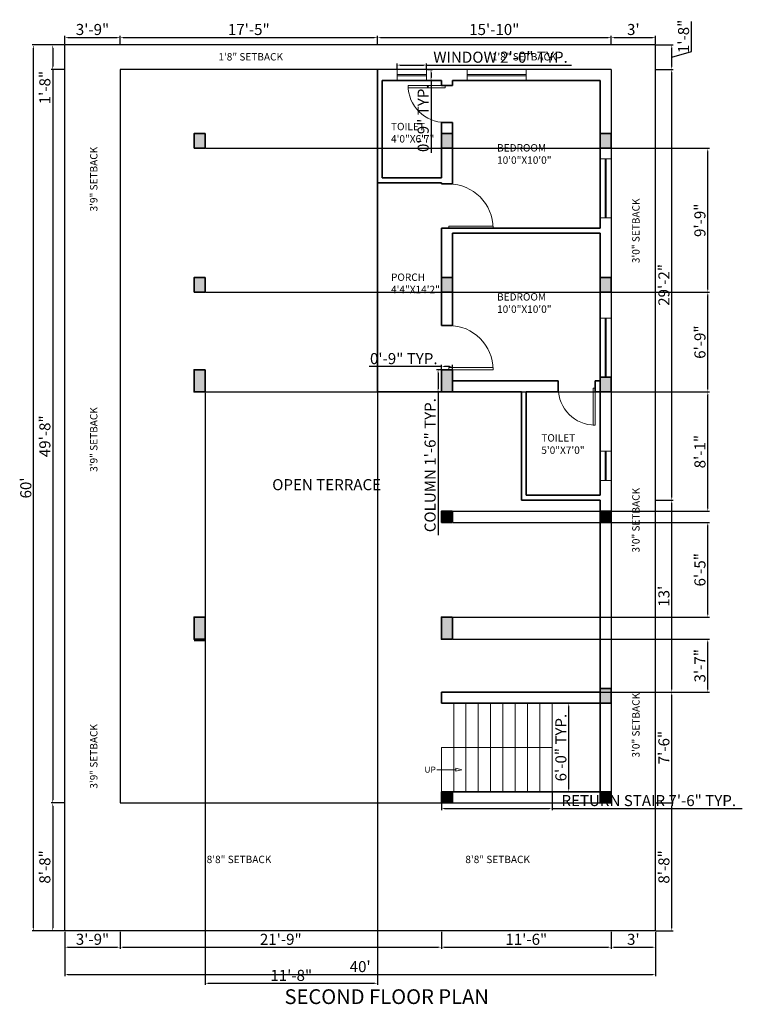
# Model space of a CAD drawing. Units: inches. Extents: x 3321 to 5237, y 11 to 1752.
# Tile 24 of 43: x 4649 to 5237, y 11 to 811. Entities that reach past the tile are written whole.
import ezdxf

# ---------------------------------------------------------------- set-up
doc = ezdxf.new("R2010")
doc.units = ezdxf.units.IN
for name, color, linetype, lineweight in [('A-ANNO-DIMS', 2, 'Continuous', 18), ('A-ANNO-SYMB', 7, 'Continuous', 18), ('A-ANNO-TEXT', 7, 'Continuous', 18), ('A-ANNO-TITL', 7, 'Continuous', 25), ('A-AREA-IDEN', 7, 'Continuous', 18), ('A-COLS', 1, 'Continuous', 35), ('A-DOOR', 4, 'Continuous', 18), ('A-FLOR-EDGE', 7, 'Continuous', 25), ('A-FLOR-STRS', 7, 'Continuous', 18), ('A-GLAZ', 5, 'Continuous', 18), ('A-WALL', 7, 'Continuous', 35), ('C-PROP', 7, 'Continuous', 30)]:
    doc.layers.add(name, color=color, linetype=linetype, lineweight=lineweight)
doc.styles.get("Standard").update_dxf_attribs({"font": 'arial.ttf'})
doc.dimstyles.new('ISO-25', dxfattribs={"dimtxt": 9, "dimasz": 2.5, "dimexe": 1.25, "dimexo": 0.625, "dimtad": 1, "dimdec": 1, "dimlunit": 3, "dimtxsty": 'Standard', "dimcen": 2.5, "dimclrd": 4, "dimclre": 4, "dimclrt": 256, "dimadec": 0, "dimazin": 0, "dimtfac": 1, "dimtdec": 1, "dimtmove": 0, "dimatfit": 3, "dimfxl": 1, "dimarcsym": 0})

# ---------------------------------------------------------------- blocks, each defined once
blk = doc.blocks.new('*U4')
for p, q in [((0, 0), (0, -6)), ((-36, 0), (-36, -6))]:
    blk.add_line(p, q)
blk.add_lwpolyline([(0, 0), (0, 36), (-1.75, 36), (-1.75, 0)], close=True)
blk.add_arc((0, 0), 36, 90, 180)
blk = doc.blocks.new('*U7')
for p, q in [((0, 0), (0, 6)), ((30, 0), (30, 6))]:
    blk.add_line(p, q)
blk.add_lwpolyline([(0, 0), (0, -30), (1.75, -30), (1.75, 0)], close=True)
blk.add_arc((0, 0), 30, 270, 0)
blk = doc.blocks.new('*U8')
for p, q in [((-30, 0), (-30, 6)), ((0, 0), (0, 6))]:
    blk.add_line(p, q)
blk.add_lwpolyline([(0, 0), (0, -30), (-1.75, -30), (-1.75, 0)], close=True)
blk.add_arc((0, 0), 30, 180, 270)
blk = doc.blocks.new('*D116')
at = {"layer": 'A-ANNO-DIMS', "color": 0, "lineweight": -2, "transparency": 16777216}
for p, q in [((4686.08, 791.23), (4686.08, 798.02)), ((4688.58, 796.77), (4728.58, 796.77)), ((4731.08, 791.23), (4731.08, 798.02))]:
    blk.add_line(p, q, dxfattribs=at)
at = {"layer": 'A-ANNO-DIMS', "color": 0, "transparency": 16777216}
for points in [[(4688.58, 797.19), (4688.58, 796.35), (4686.08, 796.77)], [(4728.58, 797.19), (4728.58, 796.35), (4731.08, 796.77)]]:
    blk.add_solid(points, dxfattribs=at)
at = {"layer": 'Defpoints', "color": 0, "transparency": 16777216}
for p in [(4731.08, 796.77), (4686.08, 790.61), (4731.08, 790.61)]:
    blk.add_point(p, dxfattribs=at)
at = {"layer": 'A-ANNO-DIMS', "color": 0, "transparency": 16777216, "insert": (4708.58, 801.99), "char_height": 9, "attachment_point": 5}
blk.add_mtext('3\'-9"', dxfattribs=at)
blk = doc.blocks.new('*D105')
at = {"layer": 'A-ANNO-DIMS', "color": 0, "lineweight": -2, "transparency": 16777216}
for p, q in [((4731.08, 791.23), (4731.08, 798.02)), ((4733.58, 796.77), (4937.58, 796.77)), ((4940.08, 791.23), (4940.08, 798.02))]:
    blk.add_line(p, q, dxfattribs=at)
at = {"layer": 'A-ANNO-DIMS', "color": 0, "transparency": 16777216}
for points in [[(4733.58, 797.19), (4733.58, 796.35), (4731.08, 796.77)], [(4937.58, 797.19), (4937.58, 796.35), (4940.08, 796.77)]]:
    blk.add_solid(points, dxfattribs=at)
at = {"layer": 'Defpoints', "color": 0, "transparency": 16777216}
for p in [(4940.08, 796.77), (4731.08, 790.61), (4940.08, 790.61)]:
    blk.add_point(p, dxfattribs=at)
at = {"layer": 'A-ANNO-DIMS', "color": 0, "transparency": 16777216, "insert": (4835.58, 801.99), "char_height": 9, "attachment_point": 5}
blk.add_mtext('17\'-5"', dxfattribs=at)
blk = doc.blocks.new('*D106')
at = {"layer": 'A-ANNO-DIMS', "color": 0, "lineweight": -2, "transparency": 16777216}
for p, q in [((4940.08, 791.23), (4940.08, 798.02)), ((4942.58, 796.77), (5127.58, 796.77)), ((5130.08, 791.23), (5130.08, 798.02))]:
    blk.add_line(p, q, dxfattribs=at)
at = {"layer": 'A-ANNO-DIMS', "color": 0, "transparency": 16777216}
for points in [[(4942.58, 797.19), (4942.58, 796.35), (4940.08, 796.77)], [(5127.58, 797.19), (5127.58, 796.35), (5130.08, 796.77)]]:
    blk.add_solid(points, dxfattribs=at)
at = {"layer": 'Defpoints', "color": 0, "transparency": 16777216}
for p in [(5130.08, 796.77), (4940.08, 790.61), (5130.08, 790.61)]:
    blk.add_point(p, dxfattribs=at)
at = {"layer": 'A-ANNO-DIMS', "color": 0, "transparency": 16777216, "insert": (5035.08, 801.99), "char_height": 9, "attachment_point": 5}
blk.add_mtext('15\'-10"', dxfattribs=at)
blk = doc.blocks.new('*D117')
at = {"layer": 'A-ANNO-DIMS', "color": 0, "lineweight": -2, "transparency": 16777216}
for p, q in [((5130.08, 791.23), (5130.08, 798.02)), ((5132.58, 796.77), (5163.58, 796.77)), ((5166.08, 791.23), (5166.08, 798.02))]:
    blk.add_line(p, q, dxfattribs=at)
at = {"layer": 'A-ANNO-DIMS', "color": 0, "transparency": 16777216}
for points in [[(5132.58, 797.19), (5132.58, 796.35), (5130.08, 796.77)], [(5163.58, 797.19), (5163.58, 796.35), (5166.08, 796.77)]]:
    blk.add_solid(points, dxfattribs=at)
at = {"layer": 'Defpoints', "color": 0, "transparency": 16777216}
for p in [(5166.08, 796.77), (5130.08, 790.61), (5166.08, 790.61)]:
    blk.add_point(p, dxfattribs=at)
at = {"layer": 'A-ANNO-DIMS', "color": 0, "transparency": 16777216, "insert": (5148.08, 801.99), "char_height": 9, "attachment_point": 5}
blk.add_mtext("3'", dxfattribs=at)
blk = doc.blocks.new('*D107')
at = {"layer": 'A-ANNO-DIMS', "color": 0, "lineweight": -2, "transparency": 16777216}
for p, q in [((4685.46, 790.61), (4674.99, 790.61)), ((4676.24, 788.11), (4676.24, 773.11)), ((4685.46, 770.61), (4674.99, 770.61)), ((4676.24, 770.61), (4676.24, 743.78))]:
    blk.add_line(p, q, dxfattribs=at)
at = {"layer": 'A-ANNO-DIMS', "color": 0, "transparency": 16777216}
for points in [[(4675.82, 788.11), (4676.66, 788.11), (4676.24, 790.61)], [(4675.82, 773.11), (4676.66, 773.11), (4676.24, 770.61)]]:
    blk.add_solid(points, dxfattribs=at)
at = {"layer": 'Defpoints', "color": 0, "transparency": 16777216}
for p in [(4686.08, 790.61), (4676.24, 770.61), (4686.08, 770.61)]:
    blk.add_point(p, dxfattribs=at)
at = {"layer": 'A-ANNO-DIMS', "color": 0, "transparency": 16777216, "insert": (4671.02, 755.94), "char_height": 9, "attachment_point": 5, "rotation": 90}
blk.add_mtext('1\'-8"', dxfattribs=at)
blk = doc.blocks.new('*D108')
at = {"layer": 'A-ANNO-DIMS', "color": 0, "lineweight": -2, "transparency": 16777216}
for p, q in [((4685.46, 770.61), (4674.99, 770.61)), ((4676.24, 768.11), (4676.24, 177.11)), ((4685.46, 174.61), (4674.99, 174.61))]:
    blk.add_line(p, q, dxfattribs=at)
at = {"layer": 'A-ANNO-DIMS', "color": 0, "transparency": 16777216}
for points in [[(4675.82, 768.11), (4676.66, 768.11), (4676.24, 770.61)], [(4675.82, 177.11), (4676.66, 177.11), (4676.24, 174.61)]]:
    blk.add_solid(points, dxfattribs=at)
at = {"layer": 'Defpoints', "color": 0, "transparency": 16777216}
for p in [(4686.08, 770.61), (4676.24, 174.61), (4686.08, 174.61)]:
    blk.add_point(p, dxfattribs=at)
at = {"layer": 'A-ANNO-DIMS', "color": 0, "transparency": 16777216, "insert": (4671.02, 472.61), "char_height": 9, "attachment_point": 5, "rotation": 90}
blk.add_mtext('49\'-8"', dxfattribs=at)
blk = doc.blocks.new('*D118')
at = {"layer": 'A-ANNO-DIMS', "color": 0, "lineweight": -2, "transparency": 16777216}
for p, q in [((4685.46, 174.61), (4674.99, 174.61)), ((4676.24, 172.11), (4676.24, 73.11)), ((4685.46, 70.61), (4674.99, 70.61))]:
    blk.add_line(p, q, dxfattribs=at)
at = {"layer": 'A-ANNO-DIMS', "color": 0, "transparency": 16777216}
for points in [[(4675.82, 172.11), (4676.66, 172.11), (4676.24, 174.61)], [(4675.82, 73.11), (4676.66, 73.11), (4676.24, 70.61)]]:
    blk.add_solid(points, dxfattribs=at)
at = {"layer": 'Defpoints', "color": 0, "transparency": 16777216}
for p in [(4686.08, 174.61), (4676.24, 70.61), (4686.08, 70.61)]:
    blk.add_point(p, dxfattribs=at)
at = {"layer": 'A-ANNO-DIMS', "color": 0, "transparency": 16777216, "insert": (4671.02, 122.61), "char_height": 9, "attachment_point": 5, "rotation": 90}
blk.add_mtext('8\'-8"', dxfattribs=at)
blk = doc.blocks.new('*D119')
at = {"layer": 'A-ANNO-DIMS', "color": 0, "lineweight": -2, "transparency": 16777216}
for p, q in [((5166.71, 174.61), (5180.54, 174.61)), ((5179.29, 73.11), (5179.29, 172.11)), ((5166.71, 70.61), (5180.54, 70.61))]:
    blk.add_line(p, q, dxfattribs=at)
at = {"layer": 'A-ANNO-DIMS', "color": 0, "transparency": 16777216}
for points in [[(5178.88, 172.11), (5179.71, 172.11), (5179.29, 174.61)], [(5178.88, 73.11), (5179.71, 73.11), (5179.29, 70.61)]]:
    blk.add_solid(points, dxfattribs=at)
at = {"layer": 'Defpoints', "color": 0, "transparency": 16777216}
for p in [(5166.08, 174.61), (5179.29, 174.61), (5166.08, 70.61)]:
    blk.add_point(p, dxfattribs=at)
at = {"layer": 'A-ANNO-DIMS', "color": 0, "transparency": 16777216, "insert": (5174.07, 122.61), "char_height": 9, "attachment_point": 5, "rotation": 90}
blk.add_mtext('8\'-8"', dxfattribs=at)
blk = doc.blocks.new('*D109')
at = {"layer": 'A-ANNO-DIMS', "color": 0, "lineweight": -2, "transparency": 16777216}
for p, q in [((5166.71, 264.61), (5180.54, 264.61)), ((5179.29, 177.11), (5179.29, 262.11)), ((5166.71, 174.61), (5180.54, 174.61))]:
    blk.add_line(p, q, dxfattribs=at)
at = {"layer": 'A-ANNO-DIMS', "color": 0, "transparency": 16777216}
for points in [[(5178.88, 262.11), (5179.71, 262.11), (5179.29, 264.61)], [(5178.88, 177.11), (5179.71, 177.11), (5179.29, 174.61)]]:
    blk.add_solid(points, dxfattribs=at)
at = {"layer": 'Defpoints', "color": 0, "transparency": 16777216}
for p in [(5166.08, 264.61), (5179.29, 264.61), (5166.08, 174.61)]:
    blk.add_point(p, dxfattribs=at)
at = {"layer": 'A-ANNO-DIMS', "color": 0, "transparency": 16777216, "insert": (5174.07, 219.61), "char_height": 9, "attachment_point": 5, "rotation": 90}
blk.add_mtext('7\'-6"', dxfattribs=at)
blk = doc.blocks.new('*D110')
at = {"layer": 'A-ANNO-DIMS', "color": 0, "lineweight": -2, "transparency": 16777216}
for p, q in [((5166.71, 420.61), (5180.54, 420.61)), ((5179.29, 267.11), (5179.29, 418.11)), ((5166.71, 264.61), (5180.54, 264.61))]:
    blk.add_line(p, q, dxfattribs=at)
at = {"layer": 'A-ANNO-DIMS', "color": 0, "transparency": 16777216}
for points in [[(5178.88, 418.11), (5179.71, 418.11), (5179.29, 420.61)], [(5178.88, 267.11), (5179.71, 267.11), (5179.29, 264.61)]]:
    blk.add_solid(points, dxfattribs=at)
at = {"layer": 'Defpoints', "color": 0, "transparency": 16777216}
for p in [(5166.08, 420.61), (5179.29, 420.61), (5166.08, 264.61)]:
    blk.add_point(p, dxfattribs=at)
at = {"layer": 'A-ANNO-DIMS', "color": 0, "transparency": 16777216, "insert": (5174.07, 342.61), "char_height": 9, "attachment_point": 5, "rotation": 90}
blk.add_mtext("13'", dxfattribs=at)
blk = doc.blocks.new('*D111')
at = {"layer": 'A-ANNO-DIMS', "color": 0, "lineweight": -2, "transparency": 16777216}
for p, q in [((5166.71, 770.61), (5180.54, 770.61)), ((5179.29, 423.11), (5179.29, 768.11)), ((5166.71, 420.61), (5180.54, 420.61))]:
    blk.add_line(p, q, dxfattribs=at)
at = {"layer": 'A-ANNO-DIMS', "color": 0, "transparency": 16777216}
for points in [[(5178.88, 768.11), (5179.71, 768.11), (5179.29, 770.61)], [(5178.88, 423.11), (5179.71, 423.11), (5179.29, 420.61)]]:
    blk.add_solid(points, dxfattribs=at)
at = {"layer": 'Defpoints', "color": 0, "transparency": 16777216}
for p in [(5166.08, 770.61), (5179.29, 770.61), (5166.08, 420.61)]:
    blk.add_point(p, dxfattribs=at)
at = {"layer": 'A-ANNO-DIMS', "color": 0, "transparency": 16777216, "insert": (5174.07, 595.61), "char_height": 9, "attachment_point": 5, "rotation": 90}
blk.add_mtext('29\'-2"', dxfattribs=at)
blk = doc.blocks.new('*D112')
at = {"layer": 'A-ANNO-DIMS', "color": 0, "lineweight": -2, "transparency": 16777216}
for p, q in [((5195.27, 785.4), (5195.27, 809.73)), ((5166.71, 790.61), (5180.54, 790.61)), ((5179.29, 773.11), (5179.29, 788.11)), ((5179.29, 780.61), (5195.27, 785.4)), ((5166.71, 770.61), (5180.54, 770.61))]:
    blk.add_line(p, q, dxfattribs=at)
at = {"layer": 'A-ANNO-DIMS', "color": 0, "transparency": 16777216}
for points in [[(5178.88, 788.11), (5179.71, 788.11), (5179.29, 790.61)], [(5178.88, 773.11), (5179.71, 773.11), (5179.29, 770.61)]]:
    blk.add_solid(points, dxfattribs=at)
at = {"layer": 'Defpoints', "color": 0, "transparency": 16777216}
for p in [(5166.08, 790.61), (5179.29, 790.61), (5166.08, 770.61)]:
    blk.add_point(p, dxfattribs=at)
at = {"layer": 'A-ANNO-DIMS', "color": 0, "transparency": 16777216, "insert": (5190.05, 797.56), "char_height": 9, "attachment_point": 5, "rotation": 90}
blk.add_mtext('1\'-8"', dxfattribs=at)
blk = doc.blocks.new('*D120')
at = {"layer": 'A-ANNO-DIMS', "color": 0, "lineweight": -2, "transparency": 16777216}
for p, q in [((4686.08, 69.98), (4686.08, 56.17)), ((4731.08, 69.98), (4731.08, 56.17)), ((4688.58, 57.42), (4728.58, 57.42))]:
    blk.add_line(p, q, dxfattribs=at)
at = {"layer": 'A-ANNO-DIMS', "color": 0, "transparency": 16777216}
for points in [[(4688.58, 57.84), (4688.58, 57.01), (4686.08, 57.42)], [(4728.58, 57.84), (4728.58, 57.01), (4731.08, 57.42)]]:
    blk.add_solid(points, dxfattribs=at)
at = {"layer": 'Defpoints', "color": 0, "transparency": 16777216}
for p in [(4686.08, 70.61), (4731.08, 70.61), (4731.08, 57.42)]:
    blk.add_point(p, dxfattribs=at)
at = {"layer": 'A-ANNO-DIMS', "color": 0, "transparency": 16777216, "insert": (4708.58, 62.65), "char_height": 9, "attachment_point": 5}
blk.add_mtext('3\'-9"', dxfattribs=at)
blk = doc.blocks.new('*D113')
at = {"layer": 'A-ANNO-DIMS', "color": 0, "lineweight": -2, "transparency": 16777216}
for p, q in [((4731.08, 69.98), (4731.08, 56.17)), ((4992.08, 69.98), (4992.08, 56.17)), ((4733.58, 57.42), (4989.58, 57.42))]:
    blk.add_line(p, q, dxfattribs=at)
at = {"layer": 'A-ANNO-DIMS', "color": 0, "transparency": 16777216}
for points in [[(4733.58, 57.84), (4733.58, 57.01), (4731.08, 57.42)], [(4989.58, 57.84), (4989.58, 57.01), (4992.08, 57.42)]]:
    blk.add_solid(points, dxfattribs=at)
at = {"layer": 'Defpoints', "color": 0, "transparency": 16777216}
for p in [(4731.08, 70.61), (4992.08, 70.61), (4992.08, 57.42)]:
    blk.add_point(p, dxfattribs=at)
at = {"layer": 'A-ANNO-DIMS', "color": 0, "transparency": 16777216, "insert": (4861.58, 62.64), "char_height": 9, "attachment_point": 5}
blk.add_mtext('21\'-9"', dxfattribs=at)
blk = doc.blocks.new('*D114')
at = {"layer": 'A-ANNO-DIMS', "color": 0, "lineweight": -2, "transparency": 16777216}
for p, q in [((4992.08, 69.98), (4992.08, 56.17)), ((5130.08, 69.98), (5130.08, 56.17)), ((4994.58, 57.42), (5127.58, 57.42))]:
    blk.add_line(p, q, dxfattribs=at)
at = {"layer": 'A-ANNO-DIMS', "color": 0, "transparency": 16777216}
for points in [[(4994.58, 57.84), (4994.58, 57.01), (4992.08, 57.42)], [(5127.58, 57.84), (5127.58, 57.01), (5130.08, 57.42)]]:
    blk.add_solid(points, dxfattribs=at)
at = {"layer": 'Defpoints', "color": 0, "transparency": 16777216}
for p in [(4992.08, 70.61), (5130.08, 70.61), (5130.08, 57.42)]:
    blk.add_point(p, dxfattribs=at)
at = {"layer": 'A-ANNO-DIMS', "color": 0, "transparency": 16777216, "insert": (5061.08, 62.64), "char_height": 9, "attachment_point": 5}
blk.add_mtext('11\'-6"', dxfattribs=at)
blk = doc.blocks.new('*D121')
at = {"layer": 'A-ANNO-DIMS', "color": 0, "lineweight": -2, "transparency": 16777216}
for p, q in [((5130.08, 69.98), (5130.08, 56.17)), ((5166.08, 69.98), (5166.08, 56.17)), ((5132.58, 57.42), (5163.58, 57.42))]:
    blk.add_line(p, q, dxfattribs=at)
at = {"layer": 'A-ANNO-DIMS', "color": 0, "transparency": 16777216}
for points in [[(5132.58, 57.84), (5132.58, 57.01), (5130.08, 57.42)], [(5163.58, 57.84), (5163.58, 57.01), (5166.08, 57.42)]]:
    blk.add_solid(points, dxfattribs=at)
at = {"layer": 'Defpoints', "color": 0, "transparency": 16777216}
for p in [(5130.08, 70.61), (5166.08, 70.61), (5166.08, 57.42)]:
    blk.add_point(p, dxfattribs=at)
at = {"layer": 'A-ANNO-DIMS', "color": 0, "transparency": 16777216, "insert": (5148.08, 62.65), "char_height": 9, "attachment_point": 5}
blk.add_mtext("3'", dxfattribs=at)
blk = doc.blocks.new('*D115')
at = {"layer": 'A-ANNO-DIMS', "color": 0, "lineweight": -2, "transparency": 16777216}
for p, q in [((4686.08, 69.98), (4686.08, 34)), ((5166.08, 69.98), (5166.08, 34)), ((4688.58, 35.25), (5163.58, 35.25))]:
    blk.add_line(p, q, dxfattribs=at)
at = {"layer": 'A-ANNO-DIMS', "color": 0, "transparency": 16777216}
for points in [[(4688.58, 35.67), (4688.58, 34.83), (4686.08, 35.25)], [(5163.58, 35.67), (5163.58, 34.83), (5166.08, 35.25)]]:
    blk.add_solid(points, dxfattribs=at)
at = {"layer": 'Defpoints', "color": 0, "transparency": 16777216}
for p in [(4686.08, 70.61), (5166.08, 70.61), (5166.08, 35.25)]:
    blk.add_point(p, dxfattribs=at)
at = {"layer": 'A-ANNO-DIMS', "color": 0, "transparency": 16777216, "insert": (4926.08, 40.47), "char_height": 9, "attachment_point": 5}
blk.add_mtext("40'", dxfattribs=at)
blk = doc.blocks.new('*D122')
at = {"layer": 'A-ANNO-DIMS', "color": 0, "lineweight": -2, "transparency": 16777216}
for p, q in [((4685.46, 790.61), (4659.51, 790.61)), ((4660.76, 73.11), (4660.76, 788.11)), ((4685.46, 70.61), (4659.51, 70.61))]:
    blk.add_line(p, q, dxfattribs=at)
at = {"layer": 'A-ANNO-DIMS', "color": 0, "transparency": 16777216}
for points in [[(4660.35, 788.11), (4661.18, 788.11), (4660.76, 790.61)], [(4660.35, 73.11), (4661.18, 73.11), (4660.76, 70.61)]]:
    blk.add_solid(points, dxfattribs=at)
at = {"layer": 'Defpoints', "color": 0, "transparency": 16777216}
for p in [(4660.76, 790.61), (4686.08, 790.61), (4686.08, 70.61)]:
    blk.add_point(p, dxfattribs=at)
at = {"layer": 'A-ANNO-DIMS', "color": 0, "transparency": 16777216, "insert": (4655.54, 430.61), "char_height": 9, "attachment_point": 5, "rotation": 90}
blk.add_mtext("60'", dxfattribs=at)
blk = doc.blocks.new('COL-9X18-IN')
h = blk.add_hatch(color=256)
h.dxf.hatch_style = 1
h.paths.add_polyline_path([(9, 18), (0, 18), (0, 0), (9, 0)])
blk.add_lwpolyline([(0, 0), (9, 0), (9, 18), (0, 18)], close=True)
blk = doc.blocks.new('COL-9X12-BASE-PLAN')
h = blk.add_hatch(color=256)
h.dxf.hatch_style = 1
h.paths.add_polyline_path([(0, 0), (9, 0), (9, 12), (0, 12)])
blk.add_lwpolyline([(0, 0), (9, 0), (9, 12), (0, 12)], close=True)
blk = doc.blocks.new('COL-9X9-BASE-PLAN')
h = blk.add_hatch(color=256)
h.dxf.hatch_style = 1
h.paths.add_polyline_path([(0, 0), (9, 0), (9, 9), (0, 9)])
blk.add_lwpolyline([(0, 0), (9, 0), (9, 9), (0, 9)], close=True)
blk = doc.blocks.new('WIN-48IN-9IN-WALL')
for p, q in [((0, 0), (0, 9)), ((48, 0), (48, 9)), ((0, 5), (48, 5)), ((0, 4), (48, 4))]:
    blk.add_line(p, q)
blk = doc.blocks.new('WIN-24IN-9IN-WALL')
for p, q in [((9, 24), (0, 24)), ((4, 24), (4, 0)), ((5, 24), (5, 0)), ((9, 0), (0, 0))]:
    blk.add_line(p, q)
blk = doc.blocks.new('STAIR-RETURN-72IN')
for p, q in [((10, 72), (10, 0)), ((20, 72), (20, 0)), ((30, 72), (30, 0)), ((40, 72), (40, 0)), ((50, 72), (50, 0)), ((60, 72), (60, 0)), ((70, 72), (70, 0)), ((80, 72), (80, 0)), ((90, 72), (90, 0)), ((90, 36), (0, 36)), ((0, 36), (0, 0))]:
    blk.add_line(p, q)
blk = doc.blocks.new('STAIR-DIRECTION-ARROW')
blk.add_line((0, 1.22), (15.43, 1.22))
blk.add_lwpolyline([(20.27, 1.22), (15.43, 2.43), (15.43, 0)], close=True)
blk = doc.blocks.new('PROPERTY-40X60FT')
for p, q in [((0, 720), (480, 720)), ((0, 720), (0, 0)), ((480, 720), (480, 0)), ((0, 0), (480, 0))]:
    blk.add_line(p, q)
blk = doc.blocks.new('*D167')
at = {"layer": 'A-ANNO-DIMS', "color": 4, "lineweight": -2, "transparency": 16777216}
for p, q in [((4956.08, 771.23), (4956.08, 775.46)), ((4958.58, 774.21), (4977.58, 774.21)), ((4980.08, 771.23), (4980.08, 775.46)), ((4980.08, 774.21), (5097.72, 774.21))]:
    blk.add_line(p, q, dxfattribs=at)
at = {"layer": 'A-ANNO-DIMS', "color": 4, "transparency": 16777216}
for points in [[(4958.58, 774.62), (4958.58, 773.79), (4956.08, 774.21)], [(4977.58, 774.62), (4977.58, 773.79), (4980.08, 774.21)]]:
    blk.add_solid(points, dxfattribs=at)
at = {"layer": 'Defpoints', "color": 0, "transparency": 16777216}
for p in [(4956.08, 770.61), (4980.08, 774.21), (4980.08, 770.61)]:
    blk.add_point(p, dxfattribs=at)
at = {"layer": 'A-ANNO-DIMS', "transparency": 16777216, "insert": (5040.15, 779.49), "char_height": 9, "attachment_point": 5}
blk.add_mtext('WINDOW 2\'-0" TYP.', dxfattribs=at)
blk = doc.blocks.new('*D168')
at = {"layer": 'A-ANNO-DIMS', "color": 4, "lineweight": -2, "transparency": 16777216}
for p, q in [((4980.71, 770.61), (4984.93, 770.61)), ((4980.71, 761.61), (4984.93, 761.61)), ((4983.68, 768.11), (4983.68, 764.11)), ((4983.68, 761.61), (4983.68, 703))]:
    blk.add_line(p, q, dxfattribs=at)
at = {"layer": 'A-ANNO-DIMS', "color": 4, "transparency": 16777216}
for points in [[(4983.27, 768.11), (4984.1, 768.11), (4983.68, 770.61)], [(4983.27, 764.11), (4984.1, 764.11), (4983.68, 761.61)]]:
    blk.add_solid(points, dxfattribs=at)
at = {"layer": 'Defpoints', "color": 0, "transparency": 16777216}
for p in [(4980.08, 770.61), (4980.08, 761.61), (4983.68, 761.61)]:
    blk.add_point(p, dxfattribs=at)
at = {"layer": 'A-ANNO-DIMS', "transparency": 16777216, "insert": (4978.46, 731.05), "char_height": 9, "attachment_point": 5, "rotation": 90}
blk.add_mtext('0\'-9" TYP.', dxfattribs=at)
blk = doc.blocks.new('*D175')
at = {"layer": 'A-ANNO-DIMS', "color": 4, "lineweight": -2, "transparency": 16777216}
for p, q in [((4991.46, 526.61), (4988.13, 526.61)), ((4989.38, 524.11), (4989.38, 511.11)), ((4991.46, 508.61), (4988.13, 508.61)), ((4989.38, 508.61), (4989.38, 392.13))]:
    blk.add_line(p, q, dxfattribs=at)
at = {"layer": 'A-ANNO-DIMS', "color": 4, "transparency": 16777216}
for points in [[(4988.97, 524.11), (4989.8, 524.11), (4989.38, 526.61)], [(4988.97, 511.11), (4989.8, 511.11), (4989.38, 508.61)]]:
    blk.add_solid(points, dxfattribs=at)
at = {"layer": 'Defpoints', "color": 0, "transparency": 16777216}
for p in [(4992.08, 526.61), (4989.38, 508.61), (4992.08, 508.61)]:
    blk.add_point(p, dxfattribs=at)
at = {"layer": 'A-ANNO-DIMS', "transparency": 16777216, "insert": (4984.1, 449.12), "char_height": 9, "attachment_point": 5, "rotation": 90}
blk.add_mtext('COLUMN 1\'-6" TYP.', dxfattribs=at)
blk = doc.blocks.new('*D176')
at = {"layer": 'A-ANNO-DIMS', "color": 4, "lineweight": -2, "transparency": 16777216}
for p, q in [((4992.08, 529.31), (4933.47, 529.31)), ((4992.08, 527.23), (4992.08, 530.56)), ((4998.58, 529.31), (4994.58, 529.31)), ((5001.08, 527.23), (5001.08, 530.56))]:
    blk.add_line(p, q, dxfattribs=at)
at = {"layer": 'A-ANNO-DIMS', "color": 4, "transparency": 16777216}
for points in [[(4994.58, 529.72), (4994.58, 528.89), (4992.08, 529.31)], [(4998.58, 529.72), (4998.58, 528.89), (5001.08, 529.31)]]:
    blk.add_solid(points, dxfattribs=at)
at = {"layer": 'Defpoints', "color": 0, "transparency": 16777216}
for p in [(4992.08, 529.31), (4992.08, 526.61), (5001.08, 526.61)]:
    blk.add_point(p, dxfattribs=at)
at = {"layer": 'A-ANNO-DIMS', "transparency": 16777216, "insert": (4961.53, 534.53), "char_height": 9, "attachment_point": 5}
blk.add_mtext('0\'-9" TYP.', dxfattribs=at)
blk = doc.blocks.new('*D189')
at = {"layer": 'A-ANNO-DIMS', "color": 4, "lineweight": -2, "transparency": 16777216}
for p, q in [((4992.08, 182.98), (4992.08, 168.86)), ((5082.08, 182.98), (5082.08, 168.86)), ((4994.58, 170.11), (5079.58, 170.11)), ((5082.08, 170.11), (5236.62, 170.11))]:
    blk.add_line(p, q, dxfattribs=at)
at = {"layer": 'A-ANNO-DIMS', "color": 4, "transparency": 16777216}
for points in [[(4994.58, 170.52), (4994.58, 169.69), (4992.08, 170.11)], [(5079.58, 170.52), (5079.58, 169.69), (5082.08, 170.11)]]:
    blk.add_solid(points, dxfattribs=at)
at = {"layer": 'Defpoints', "color": 0, "transparency": 16777216}
for p in [(4992.08, 183.61), (5082.08, 183.61), (5082.08, 170.11)]:
    blk.add_point(p, dxfattribs=at)
at = {"layer": 'A-ANNO-DIMS', "transparency": 16777216, "insert": (5160.6, 175.39), "char_height": 9, "attachment_point": 5}
blk.add_mtext('RETURN STAIR 7\'-6" TYP.', dxfattribs=at)
blk = doc.blocks.new('*D190')
at = {"layer": 'A-ANNO-DIMS', "color": 4, "lineweight": -2, "transparency": 16777216}
for p, q in [((5082.71, 255.61), (5096.83, 255.61)), ((5095.58, 186.11), (5095.58, 253.11)), ((5082.71, 183.61), (5096.83, 183.61))]:
    blk.add_line(p, q, dxfattribs=at)
at = {"layer": 'A-ANNO-DIMS', "color": 4, "transparency": 16777216}
for points in [[(5095.17, 253.11), (5096, 253.11), (5095.58, 255.61)], [(5095.17, 186.11), (5096, 186.11), (5095.58, 183.61)]]:
    blk.add_solid(points, dxfattribs=at)
at = {"layer": 'Defpoints', "color": 0, "transparency": 16777216}
for p in [(5082.08, 255.61), (5095.58, 255.61), (5082.08, 183.61)]:
    blk.add_point(p, dxfattribs=at)
at = {"layer": 'A-ANNO-DIMS', "transparency": 16777216, "insert": (5090.36, 219.61), "char_height": 9, "attachment_point": 5, "rotation": 90}
blk.add_mtext('6\'-0" TYP.', dxfattribs=at)
blk = doc.blocks.new('*D227')
at = {"layer": 'A-ANNO-DIMS', "color": 4, "lineweight": -2, "transparency": 16777216}
for p, q in [((4800.08, 507.98), (4800.08, 26.86)), ((4940.08, 507.98), (4940.08, 26.86)), ((4802.58, 28.11), (4937.58, 28.11))]:
    blk.add_line(p, q, dxfattribs=at)
at = {"layer": 'A-ANNO-DIMS', "color": 4, "transparency": 16777216}
for points in [[(4802.58, 28.52), (4802.58, 27.69), (4800.08, 28.11)], [(4937.58, 28.52), (4937.58, 27.69), (4940.08, 28.11)]]:
    blk.add_solid(points, dxfattribs=at)
at = {"layer": 'Defpoints', "color": 0, "transparency": 16777216}
for p in [(4800.08, 508.61), (4940.08, 508.61), (4940.08, 28.11)]:
    blk.add_point(p, dxfattribs=at)
at = {"layer": 'A-ANNO-DIMS', "transparency": 16777216, "insert": (4870.08, 33.33), "char_height": 9, "attachment_point": 5}
blk.add_mtext('11\'-8"', dxfattribs=at)
blk = doc.blocks.new('*D228')
at = {"layer": 'A-ANNO-DIMS', "color": 4, "lineweight": -2, "transparency": 16777216}
for p, q in [((5001.71, 307.61), (5209.83, 307.61)), ((5208.58, 267.11), (5208.58, 305.11)), ((4992.71, 264.61), (5209.83, 264.61))]:
    blk.add_line(p, q, dxfattribs=at)
at = {"layer": 'A-ANNO-DIMS', "color": 4, "transparency": 16777216}
for points in [[(5208.17, 305.11), (5209, 305.11), (5208.58, 307.61)], [(5208.17, 267.11), (5209, 267.11), (5208.58, 264.61)]]:
    blk.add_solid(points, dxfattribs=at)
at = {"layer": 'Defpoints', "color": 0, "transparency": 16777216}
for p in [(5001.08, 307.61), (5208.58, 307.61), (4992.08, 264.61)]:
    blk.add_point(p, dxfattribs=at)
at = {"layer": 'A-ANNO-DIMS', "transparency": 16777216, "insert": (5203.36, 286.11), "char_height": 9, "attachment_point": 5, "rotation": 90}
blk.add_mtext('3\'-7"', dxfattribs=at)
blk = doc.blocks.new('*D229')
at = {"layer": 'A-ANNO-DIMS', "color": 4, "lineweight": -2, "transparency": 16777216}
for p, q in [((5001.71, 402.61), (5209.83, 402.61)), ((5208.58, 328.11), (5208.58, 400.11)), ((5001.71, 325.61), (5209.83, 325.61))]:
    blk.add_line(p, q, dxfattribs=at)
at = {"layer": 'A-ANNO-DIMS', "color": 4, "transparency": 16777216}
for points in [[(5208.17, 400.11), (5209, 400.11), (5208.58, 402.61)], [(5208.17, 328.11), (5209, 328.11), (5208.58, 325.61)]]:
    blk.add_solid(points, dxfattribs=at)
at = {"layer": 'Defpoints', "color": 0, "transparency": 16777216}
for p in [(5001.08, 402.61), (5208.58, 402.61), (5001.08, 325.61)]:
    blk.add_point(p, dxfattribs=at)
at = {"layer": 'A-ANNO-DIMS', "transparency": 16777216, "insert": (5203.36, 364.11), "char_height": 9, "attachment_point": 5, "rotation": 90}
blk.add_mtext('6\'-5"', dxfattribs=at)
blk = doc.blocks.new('*D230')
at = {"layer": 'A-ANNO-DIMS', "color": 4, "lineweight": -2, "transparency": 16777216}
for p, q in [((5001.71, 508.61), (5209.83, 508.61)), ((5208.58, 414.11), (5208.58, 506.11)), ((5001.71, 411.61), (5209.83, 411.61))]:
    blk.add_line(p, q, dxfattribs=at)
at = {"layer": 'A-ANNO-DIMS', "color": 4, "transparency": 16777216}
for points in [[(5208.17, 506.11), (5209, 506.11), (5208.58, 508.61)], [(5208.17, 414.11), (5209, 414.11), (5208.58, 411.61)]]:
    blk.add_solid(points, dxfattribs=at)
at = {"layer": 'Defpoints', "color": 0, "transparency": 16777216}
for p in [(5001.08, 508.61), (5208.58, 508.61), (5001.08, 411.61)]:
    blk.add_point(p, dxfattribs=at)
at = {"layer": 'A-ANNO-DIMS', "transparency": 16777216, "insert": (5203.36, 460.11), "char_height": 9, "attachment_point": 5, "rotation": 90}
blk.add_mtext('8\'-1"', dxfattribs=at)
blk = doc.blocks.new('*D231')
at = {"layer": 'A-ANNO-DIMS', "color": 4, "lineweight": -2, "transparency": 16777216}
for p, q in [((4800.71, 589.61), (5209.83, 589.61)), ((5208.58, 511.11), (5208.58, 587.11)), ((4800.71, 508.61), (5209.83, 508.61))]:
    blk.add_line(p, q, dxfattribs=at)
at = {"layer": 'A-ANNO-DIMS', "color": 4, "transparency": 16777216}
for points in [[(5208.17, 587.11), (5209, 587.11), (5208.58, 589.61)], [(5208.17, 511.11), (5209, 511.11), (5208.58, 508.61)]]:
    blk.add_solid(points, dxfattribs=at)
at = {"layer": 'Defpoints', "color": 0, "transparency": 16777216}
for p in [(4800.08, 589.61), (5208.58, 589.61), (4800.08, 508.61)]:
    blk.add_point(p, dxfattribs=at)
at = {"layer": 'A-ANNO-DIMS', "transparency": 16777216, "insert": (5203.36, 549.11), "char_height": 9, "attachment_point": 5, "rotation": 90}
blk.add_mtext('6\'-9"', dxfattribs=at)
blk = doc.blocks.new('*D232')
at = {"layer": 'A-ANNO-DIMS', "color": 4, "lineweight": -2, "transparency": 16777216}
for p, q in [((4800.71, 706.61), (5209.83, 706.61)), ((5208.58, 592.11), (5208.58, 704.11)), ((4800.71, 589.61), (5209.83, 589.61))]:
    blk.add_line(p, q, dxfattribs=at)
at = {"layer": 'A-ANNO-DIMS', "color": 4, "transparency": 16777216}
for points in [[(5208.17, 704.11), (5209, 704.11), (5208.58, 706.61)], [(5208.17, 592.11), (5209, 592.11), (5208.58, 589.61)]]:
    blk.add_solid(points, dxfattribs=at)
at = {"layer": 'Defpoints', "color": 0, "transparency": 16777216}
for p in [(4800.08, 706.61), (5208.58, 706.61), (4800.08, 589.61)]:
    blk.add_point(p, dxfattribs=at)
at = {"layer": 'A-ANNO-DIMS', "transparency": 16777216, "insert": (5203.36, 648.11), "char_height": 9, "attachment_point": 5, "rotation": 90}
blk.add_mtext('9\'-9"', dxfattribs=at)

msp = doc.modelspace()

# ---------------------------------------------------------------- linework, layer by layer
at = {"layer": 'A-COLS'}
for p, q in [((4791.08, 526.61), (4800.08, 526.61)), ((4800.08, 526.61), (4800.08, 517.61)), ((4791.08, 306.61), (4800.08, 306.61))]:
    msp.add_line(p, q, dxfattribs=at)
at = {"layer": 'A-FLOR-EDGE'}
for p, q in [((4731.08, 770.61), (4731.08, 174.61)), ((5130.08, 770.61), (4731.08, 770.61)), ((5130.08, 770.61), (5130.08, 174.61)), ((4731.08, 174.61), (5130.08, 174.61))]:
    msp.add_line(p, q, dxfattribs=at)
at = {"layer": 'A-WALL'}
for p, q in [((4940.08, 770.61), (4940.08, 508.61)), ((4944.08, 761.61), (4944.08, 682.61)), ((4992.08, 761.61), (4944.08, 761.61)), ((4992.08, 761.61), (4992.08, 757.61)), ((5001.08, 761.61), (5001.08, 757.61)), ((5121.08, 761.61), (5001.08, 761.61)), ((5121.08, 761.61), (5121.08, 641.61)), ((5001.08, 757.61), (4992.08, 757.61)), ((4992.08, 727.61), (4992.08, 682.61)), ((5001.08, 727.61), (4992.08, 727.61)), ((5001.08, 727.61), (5001.08, 677.61)), ((4992.08, 682.61), (4944.08, 682.61)), ((4992.08, 678.61), (4940.08, 678.61)), ((4992.08, 678.61), (4992.08, 677.61)), ((5001.08, 677.61), (4992.08, 677.61)), ((4992.08, 641.61), (4992.08, 562.61)), ((5121.08, 641.61), (4992.08, 641.61)), ((5001.08, 637.61), (5001.08, 562.61)), ((5001.08, 637.61), (5121.08, 637.61)), ((5121.08, 637.61), (5121.08, 517.61)), ((4992.08, 601.61), (5001.08, 601.61)), ((4992.08, 562.61), (5001.08, 562.61)), ((4992.08, 526.61), (5001.08, 526.61)), ((5001.08, 526.61), (5001.08, 517.61)), ((5001.08, 517.61), (5087.08, 517.61)), ((5087.08, 517.61), (5087.08, 508.61)), ((5117.08, 517.61), (5117.08, 508.61)), ((5117.08, 517.61), (5121.08, 517.61)), ((4940.08, 508.61), (5057.08, 508.61)), ((5057.08, 508.61), (5057.08, 458.61)), ((5061.08, 508.61), (5061.08, 424.61)), ((5061.08, 508.61), (5087.08, 508.61)), ((5117.08, 508.61), (5121.08, 508.61)), ((5121.08, 508.61), (5121.08, 424.61)), ((5057.08, 458.61), (5057.08, 420.61)), ((5061.08, 424.61), (5121.08, 424.61)), ((5057.08, 420.61), (5121.08, 420.61)), ((5121.08, 420.61), (5121.08, 264.61)), ((4992.08, 264.61), (5121.08, 264.61)), ((4992.08, 264.61), (4992.08, 255.61)), ((4992.08, 255.61), (5121.08, 255.61)), ((5121.08, 255.61), (5121.08, 183.61)), ((4992.08, 183.61), (4992.08, 174.61)), ((4992.08, 183.61), (5121.08, 183.61))]:
    msp.add_line(p, q, dxfattribs=at)

# ---------------------------------------------------------------- block references
at = {"layer": 'A-ANNO-SYMB'}
msp.add_blockref('STAIR-DIRECTION-ARROW', (4988.36, 200.39), dxfattribs=at)
at = {"layer": 'A-COLS'}
for name, p in [('COL-9X12-BASE-PLAN', (4791.08, 706.61)), ('COL-9X12-BASE-PLAN', (4992.08, 706.61)), ('COL-9X12-BASE-PLAN', (5121.08, 706.61)), ('COL-9X12-BASE-PLAN', (4791.08, 589.61)), ('COL-9X12-BASE-PLAN', (4992.08, 589.61)), ('COL-9X12-BASE-PLAN', (5121.08, 589.61)), ('COL-9X12-BASE-PLAN', (5121.08, 508.61)), ('COL-9X9-BASE-PLAN', (4992.08, 402.61)), ('COL-9X9-BASE-PLAN', (5121.08, 402.61)), ('COL-9X12-BASE-PLAN', (5121.08, 255.61)), ('COL-9X9-BASE-PLAN', (4992.08, 174.61)), ('COL-9X9-BASE-PLAN', (5121.08, 174.61))]:
    msp.add_blockref(name, p, dxfattribs=at)
at = {"layer": 'A-COLS', "rotation": 180}
for p in [(4800.08, 526.61), (5001.08, 526.61), (4800.08, 325.61), (5001.08, 325.61)]:
    msp.add_blockref('COL-9X18-IN', p, dxfattribs=at)
at = {"layer": 'A-DOOR', "rotation": 270}
for name, p in [('*U7', (4995.08, 757.61)), ('*U4', (4998.08, 641.61)), ('*U4', (4998.08, 526.61))]:
    msp.add_blockref(name, p, dxfattribs=at)
at = {"layer": 'A-DOOR'}
msp.add_blockref('*U8', (5117.08, 511.61), dxfattribs=at)
at = {"layer": 'A-FLOR-STRS'}
msp.add_blockref('STAIR-RETURN-72IN', (4992.08, 183.61), dxfattribs=at)
at = {"layer": 'A-GLAZ'}
for name, p, rotation in [('WIN-24IN-9IN-WALL', (4956.08, 770.61), 269.9999999999976), ('WIN-48IN-9IN-WALL', (5130.08, 650.11), 89.99999999999824), ('WIN-48IN-9IN-WALL', (5130.08, 520.61), 89.99999999999824)]:
    msp.add_blockref(name, p, dxfattribs=dict(at, rotation=rotation))
for name, p in [('WIN-48IN-9IN-WALL', (5013.06, 761.61)), ('WIN-24IN-9IN-WALL', (5121.08, 436.61))]:
    msp.add_blockref(name, p, dxfattribs=at)
at = {"layer": 'C-PROP', "rotation": 180}
msp.add_blockref('PROPERTY-40X60FT', (5166.08, 790.61), dxfattribs=at)

# ---------------------------------------------------------------- texts
at = {"layer": 'A-ANNO-TEXT'}
msp.add_text('UP', height=5, dxfattribs=at).set_placement((4978.3, 199.21))
at = {"layer": 'A-ANNO-TEXT', "char_height": 6, "attachment_point": 1}
for s, insert in [('1\'8" SETBACK', (4810.85, 783.97)), ('1\'8" SETBACK', (5033.07, 783.97)), ('8\'8" SETBACK', (4801.35, 131.73)), ('8\'8" SETBACK', (5011.54, 131.73))]:
    msp.add_mtext_dynamic_manual_height_columns(s, width=97.3114, gutter_width=25, heights=[0], dxfattribs=dict(at, insert=insert))
at = {"layer": 'A-ANNO-TEXT', "char_height": 6, "attachment_point": 1, "rotation": 90}
for s, insert in [('3\'9" SETBACK', (4706.6, 655.29)), ('3\'0" SETBACK', (5147.15, 613.28)), ('3\'9" SETBACK', (4706.6, 443.71)), ('3\'0" SETBACK', (5147.15, 378.11)), ('3\'0" SETBACK', (5147.15, 211.53)), ('3\'9" SETBACK', (4706.6, 186.23))]:
    msp.add_mtext_dynamic_manual_height_columns(s, width=97.3114, gutter_width=25, heights=[0], dxfattribs=dict(at, insert=insert))
at = {"layer": 'A-ANNO-TITL', "insert": (4864.61, 23.21), "char_height": 12, "attachment_point": 1}
msp.add_mtext_dynamic_manual_height_columns('SECOND FLOOR PLAN', width=241.3793, gutter_width=25, heights=[0], dxfattribs=at)
at = {"layer": 'A-AREA-IDEN', "attachment_point": 1}
for s, width, insert, char_height in [('TOILET\\P4\'0"X6\'7"', 97.3114, (4951.15, 727.3), 6), ('BEDROOM\\P10\'0"X10\'0"', 97.3114, (5037.34, 710.01), 6), ('PORCH\\P4\'4"X14\'2"', 97.3114, (4951.15, 604.87), 6), ('BEDROOM\\P10\'0"X10\'0"', 97.3114, (5037.34, 588.88), 6), ('TOILET\\P5\'0"X7\'0"', 97.3114, (5073.28, 474.29), 6), ('OPEN TERRACE', 123.9378, (4854.62, 437.78), 9)]:
    msp.add_mtext_dynamic_manual_height_columns(s, width=width, gutter_width=25, heights=[0], dxfattribs=dict(at, insert=insert, char_height=char_height))

# ---------------------------------------------------------------- dimensions: what is measured, and where the dimension line sits
at = {"layer": 'A-ANNO-DIMS'}
for base, p1, p2, override, picture, middle in [((5179.29, 790.61), (5166.08, 770.61), (5166.08, 790.61), {"dimclrd": 0, "dimclre": 0, "dimclrt": 0, "dimtmove": 1}, '*D112', (5190.05, 786.03)), ((4660.76, 790.61), (4686.08, 70.61), (4686.08, 790.61), {"dimclrd": 0, "dimclre": 0, "dimclrt": 0}, '*D122', (4655.54, 430.61)), ((4676.24, 770.61), (4686.08, 790.61), (4686.08, 770.61), {"dimclrd": 0, "dimclre": 0, "dimclrt": 0}, '*D107', (4671.02, 755.94)), ((4676.24, 174.61), (4686.08, 770.61), (4686.08, 174.61), {"dimclrd": 0, "dimclre": 0, "dimclrt": 0}, '*D108', (4671.02, 472.61)), ((5179.29, 770.61), (5166.08, 420.61), (5166.08, 770.61), {"dimclrd": 0, "dimclre": 0, "dimclrt": 0, "dimtmove": 1}, '*D111', (5174.07, 595.61)), ((5208.58, 706.61), (4800.08, 589.61), (4800.08, 706.61), {"dimdec": 1, "dimlfac": 1, "dimrnd": 0, "dimzin": 1, "dimdsep": 46, "dimlunit": 4, "dimfrac": 2}, '*D232', (5203.36, 648.11)), ((5208.58, 589.61), (4800.08, 508.61), (4800.08, 589.61), {"dimdec": 1, "dimlfac": 1, "dimrnd": 0, "dimzin": 1, "dimdsep": 46, "dimlunit": 4, "dimfrac": 2}, '*D231', (5203.36, 549.11)), ((5208.58, 508.61), (5001.08, 411.61), (5001.08, 508.61), {"dimdec": 1, "dimlfac": 1, "dimrnd": 0, "dimzin": 1, "dimdsep": 46, "dimlunit": 4, "dimfrac": 2}, '*D230', (5203.36, 460.11)), ((5179.29, 420.61), (5166.08, 264.61), (5166.08, 420.61), {"dimclrd": 0, "dimclre": 0, "dimclrt": 0, "dimtmove": 1}, '*D110', (5174.07, 342.61)), ((5208.58, 402.61), (5001.08, 325.61), (5001.08, 402.61), {"dimdec": 1, "dimlfac": 1, "dimrnd": 0, "dimzin": 1, "dimdsep": 46, "dimlunit": 4, "dimfrac": 2}, '*D229', (5203.36, 364.11)), ((5208.58, 307.61), (4992.08, 264.61), (5001.08, 307.61), {"dimdec": 1, "dimlfac": 1, "dimrnd": 0, "dimzin": 1, "dimdsep": 46, "dimlunit": 4, "dimfrac": 2}, '*D228', (5203.36, 286.11)), ((5179.29, 264.61), (5166.08, 174.61), (5166.08, 264.61), {"dimclrd": 0, "dimclre": 0, "dimclrt": 0, "dimtmove": 1}, '*D109', (5174.07, 219.61)), ((4676.24, 70.61), (4686.08, 174.61), (4686.08, 70.61), {"dimclrd": 0, "dimclre": 0, "dimclrt": 0}, '*D118', (4671.02, 122.61)), ((5179.29, 174.61), (5166.08, 70.61), (5166.08, 174.61), {"dimclrd": 0, "dimclre": 0, "dimclrt": 0}, '*D119', (5174.07, 122.61))]:
    dim = msp.add_linear_dim(base=base, p1=p1, p2=p2, angle=90, dimstyle='ISO-25', override=override, dxfattribs=at)
    dim.commit()
    dim.dimension.update_dxf_attribs({"geometry": picture, "text_midpoint": middle})
for base, p1, p2, override, picture, middle in [((4731.08, 796.77), (4686.08, 790.61), (4731.08, 790.61), {"dimclrd": 0, "dimclre": 0, "dimclrt": 0}, '*D116', (4708.58, 801.99)), ((4940.08, 796.77), (4731.08, 790.61), (4940.08, 790.61), {"dimclrd": 0, "dimclre": 0, "dimclrt": 0}, '*D105', (4835.58, 801.99)), ((5130.08, 796.77), (4940.08, 790.61), (5130.08, 790.61), {"dimclrd": 0, "dimclre": 0, "dimclrt": 0}, '*D106', (5035.08, 801.99)), ((5166.08, 796.77), (5130.08, 790.61), (5166.08, 790.61), {"dimclrd": 0, "dimclre": 0, "dimclrt": 0}, '*D117', (5148.08, 801.99)), ((4940.08, 28.11), (4800.08, 508.61), (4940.08, 508.61), {"dimdec": 1, "dimlfac": 1, "dimrnd": 0, "dimzin": 1, "dimdsep": 46, "dimlunit": 4, "dimfrac": 2}, '*D227', (4870.08, 33.33)), ((4731.08, 57.42), (4686.08, 70.61), (4731.08, 70.61), {"dimclrd": 0, "dimclre": 0, "dimclrt": 0}, '*D120', (4708.58, 62.65)), ((5166.08, 35.25), (4686.08, 70.61), (5166.08, 70.61), {"dimclrd": 0, "dimclre": 0, "dimclrt": 0}, '*D115', (4926.08, 40.47)), ((4992.08, 57.42), (4731.08, 70.61), (4992.08, 70.61), {"dimclrd": 0, "dimclre": 0, "dimclrt": 0, "dimtmove": 1}, '*D113', (4861.58, 62.64)), ((5130.08, 57.42), (4992.08, 70.61), (5130.08, 70.61), {"dimclrd": 0, "dimclre": 0, "dimclrt": 0, "dimtmove": 1}, '*D114', (5061.08, 62.64)), ((5166.08, 57.42), (5130.08, 70.61), (5166.08, 70.61), {"dimclrd": 0, "dimclre": 0, "dimclrt": 0, "dimtmove": 1}, '*D121', (5148.08, 62.65))]:
    dim = msp.add_linear_dim(base=base, p1=p1, p2=p2, dimstyle='ISO-25', override=override, dxfattribs=at)
    dim.commit()
    dim.dimension.update_dxf_attribs({"geometry": picture, "text_midpoint": middle})
for base, p1, p2, text, picture, middle in [((4980.08, 774.21), (4956.08, 770.61), (4980.08, 770.61), 'WINDOW <> TYP.', '*D167', (5040.15, 779.49)), ((5082.08, 170.11), (4992.08, 183.61), (5082.08, 183.61), 'RETURN STAIR <> TYP.', '*D189', (5160.6, 175.39))]:
    dim = msp.add_linear_dim(base=base, p1=p1, p2=p2, text=text, dimstyle='ISO-25', override={"dimdec": 1, "dimlfac": 1, "dimrnd": 0, "dimzin": 1, "dimdsep": 46, "dimlunit": 4, "dimfrac": 2}, dxfattribs=at)
    dim.commit()
    dim.dimension.update_dxf_attribs({"geometry": picture, "text_midpoint": middle})
for base, p1, p2, angle, text, picture, middle in [((4983.68, 761.61), (4980.08, 770.61), (4980.08, 761.61), 270, '<> TYP.', '*D168', (4978.46, 731.05)), ((4992.08, 529.31), (5001.08, 526.61), (4992.08, 526.61), 180, '<> TYP.', '*D176', (4961.53, 534.53)), ((4989.38, 508.61), (4992.08, 526.61), (4992.08, 508.61), 270, 'COLUMN <> TYP.', '*D175', (4984.1, 449.12)), ((5095.58, 255.61), (5082.08, 183.61), (5082.08, 255.61), 90, '<> TYP.', '*D190', (5090.36, 219.61))]:
    dim = msp.add_linear_dim(base=base, p1=p1, p2=p2, angle=angle, text=text, dimstyle='ISO-25', override={"dimdec": 1, "dimlfac": 1, "dimrnd": 0, "dimzin": 1, "dimdsep": 46, "dimlunit": 4, "dimfrac": 2}, dxfattribs=at)
    dim.commit()
    dim.dimension.update_dxf_attribs({"geometry": picture, "text_midpoint": middle})

doc.saveas('drawing.dxf')
